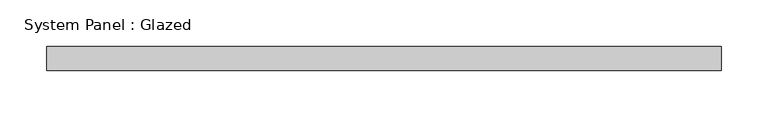
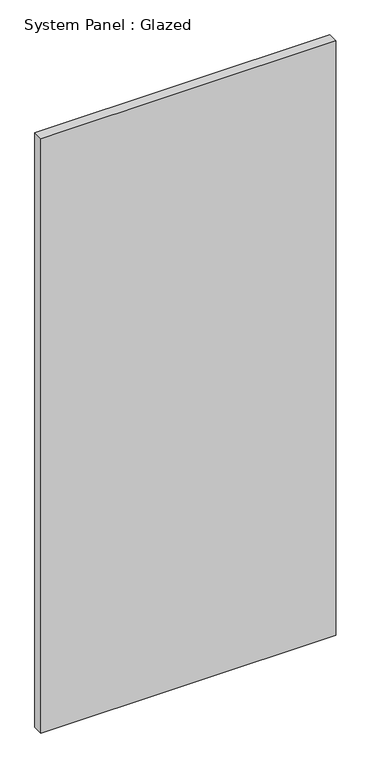
"""IFC4 building model written with IfcOpenShell, lengths in millimetres: plate geometry, System Panel : Glazed."""

from ifc_helpers import new_model, si_unit, origin, origin_with_axes, place, context, project, spatial, polyline, outline, extrude, source, transform, mapped, element, save


def system_panel_glazed_863e5c36(model_context):
    return source(origin(), model_context, "Body", "SweptSolid", [
        extrude(outline(polyline([(358.775, 19.05), (-358.775, 19.05), (-358.775, 44.45), (358.775, 44.45), (358.775, 19.05)])), origin_with_axes(), (0.0, 0.0, 1.0), 1529.4112238),
    ])


if __name__ == "__main__":
    model = new_model("IFC4")
    model_context = context("Model", 3, world=origin())
    ifc_project = project(units=[si_unit("LENGTHUNIT", "METRE", prefix="MILLI")], contexts=[model_context])
    site = spatial("IfcSite", under=ifc_project)
    building = spatial("IfcBuilding", under=site)
    placement = place(None, origin())
    system_panel_glazed_shape = system_panel_glazed_863e5c36(model_context)
    element("IfcPlate", 1, ObjectType="System Panel : Glazed", at=placement, inside=building, context=model_context, shape_type="MappedRepresentation", body=[
        mapped(system_panel_glazed_shape, transform((0.0, 0.0, 0.0), x_axis=(1.0, 0.0, 0.0), y_axis=(0.0, 1.0, 0.0), z_axis=(0.0, 0.0, 1.0))),
    ])
    save(model, "model.ifc")

# Revit data of these elements
# Type "System Panel : Glazed"
#   Construction Type Id = "GSP4R"
#   Analytic Construction = "1/8 in Pilkington single glazing"
#   Visual Light Transmittance = 0.9
#   Solar Heat Gain Coefficient = 0.86
#   Heat Transfer Coefficient (U) = 1.18115 BTU/(h·ft²·°F)
#   Define Thermal Properties by = 1
# Element 1 (IfcPlate, "System Panel : Glazed")
#   Materials on its faces: "Glass"
# Materials
#   "Glass": class "Glass", colour RGB 0 128 192, transparency 0.75, Description = "Soda Lime Glass", Cost = 0
